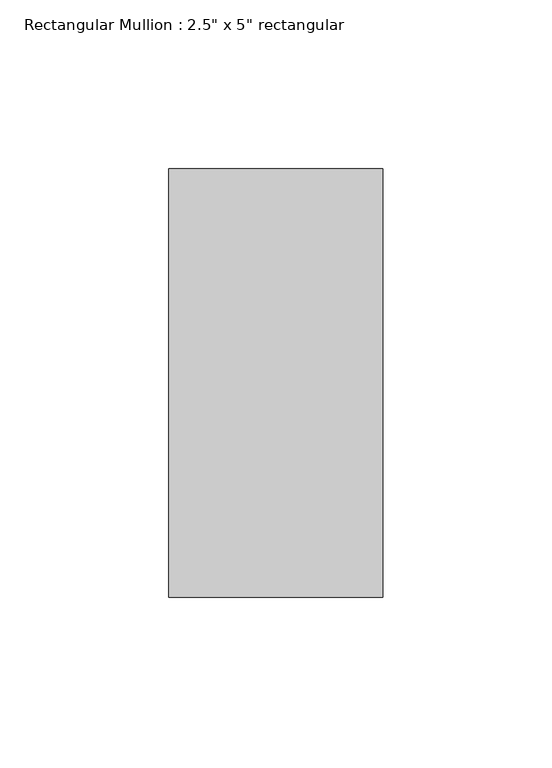
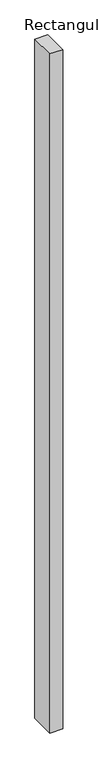
"""IFC4 building model written with IfcOpenShell, lengths in millimetres: member geometry."""

from ifc_helpers import new_model, si_unit, frame, origin, place, context, project, spatial, polyline, outline, extrude, source, transform, mapped, element, save


def member_3a1e0d67(model_context):
    return source(origin(), model_context, "Body", "SweptSolid", [
        extrude(outline(polyline([(0.0, 63.5), (0.0, -63.5), (-63.5, -63.5), (-63.5, 63.5), (0.0, 63.5)])), frame((0.0, 0.0, -3530.3050856), z_axis=(0.0, 0.0, 1.0), x_axis=(1.0, 0.0, 0.0)), (0.0, 0.0, 1.0), 3530.3050856),
    ])


if __name__ == "__main__":
    model = new_model("IFC4")
    model_context = context("Model", 3, world=origin())
    ifc_project = project(units=[si_unit("LENGTHUNIT", "METRE", prefix="MILLI")], contexts=[model_context])
    site = spatial("IfcSite", under=ifc_project)
    building = spatial("IfcBuilding", under=site)
    placement = place(None, origin())
    member_shape = member_3a1e0d67(model_context)
    element("IfcMember", 1, ObjectType="Rectangular Mullion : 2.5\" x 5\" rectangular", at=placement, inside=building, context=model_context, shape_type="MappedRepresentation", body=[
        mapped(member_shape, transform((0.0, 0.0, 0.0), x_axis=(1.0, 0.0, 0.0), y_axis=(0.0, 1.0, 0.0), z_axis=(0.0, 0.0, 1.0))),
    ])
    save(model, "model.ifc")

# Revit data of these elements
# Type "Rectangular Mullion : 2.5\" x 5\" rectangular"
#   built-in parameter 1007304 = 0.416667 (stored number, unit not read)
#   built-in parameter 1007301 = 0.104167 (stored number, unit not read)
#   built-in parameter 1007300 = 0.104167 (stored number, unit not read)
# Element 1 (IfcMember, "Rectangular Mullion : 2.5\" x 5\" rectangular")
#   Materials on its faces: "Iron, Ductile"
# Materials
#   "Iron, Ductile": class "Metal", colour RGB 0 0 0, transparency 0, Description = "Ductile cast iron", Cost = 0
